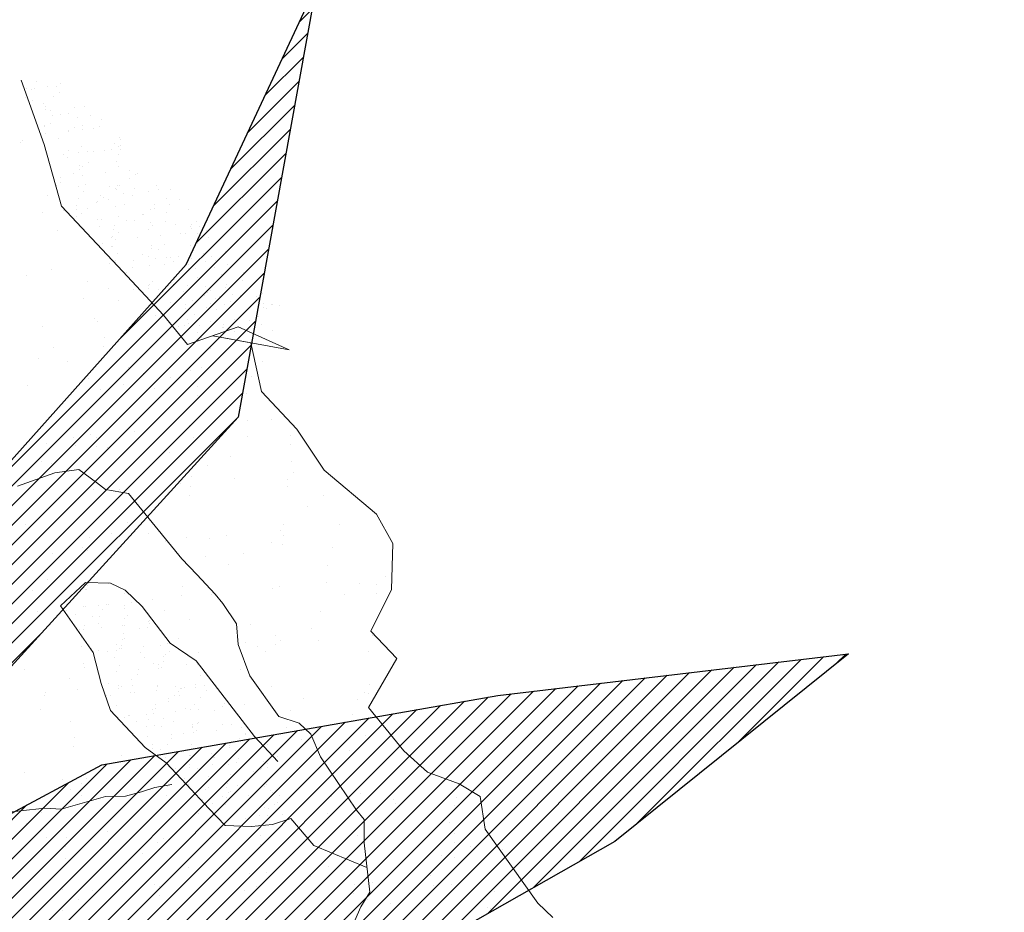
# Model space of a CAD drawing. Units: inches. Extents: x 1986 to 21484, y -1816 to 2016.
# Tile 75 of 85: x 3676.66 to 3687.55, y 1888.79 to 1898.67. Entities that reach past the tile are written whole.
import ezdxf

# ---------------------------------------------------------------- set-up
doc = ezdxf.new("R2010")
doc.units = ezdxf.units.IN
doc.layers.add('L-PLNT', color=84, linetype='Continuous', lineweight=13)
doc.layers.add('vfolhas', color=114, linetype='Continuous', lineweight=5)
doc.layers.add('vfolha2', color=110, linetype='Continuous')
doc.layers.add('vfolhas2', color=102, linetype='Continuous')
pattern_1 = [(45, (-2446.5133113, 50.986076), (-0.004419417382, 0.004419417382), [])]

# ---------------------------------------------------------------- blocks, each defined once
blk = doc.blocks.new('arbusto_PB_verde_grande')
at = {"layer": 'vfolha2'}
h = blk.add_hatch(dxfattribs=at)
h.set_pattern_fill('ANSI31', color=256, scale=0.05, style=0)
h.set_pattern_definition(pattern_1)
h.paths.add_polyline_path([(0.02944, 0.35651), (0.00028, 0.09048), (0.02625, -0.03934), (0.047, 0.06233), (0.06189, 0.09731), (0.09372, 0.26573), (0.09955, 0.43473), (0.08789, 0.61313), (0.0645, 0.72266), (0.04988, 0.6851), (0.0236, 0.51294)])
h.paths.add_polyline_path([(0.30106, 0.43789), (0.14225, 0.24871), (0.26685, 0.30022)])
h.paths.add_polyline_path([(0.37995, 0.22817), (0.23697, 0.15193), (0.18428, 0.09364), (0.11122, 0.04358), (0.02625, -0.03934), (0.28061, 0.04667), (0.36829, 0.07798), (0.46756, 0.11239), (0.61068, 0.19376), (0.71585, 0.27823), (0.55813, 0.25948)])
h.paths.add_polyline_path([(0.56101, -0.29441), (0.72752, -0.32573), (0.59024, -0.2412), (0.42962, -0.15982), (0.02625, -0.03934), (0.14922, -0.14107), (0.18838, -0.16604), (0.41501, -0.24435)])
h.paths.add_polyline_path([(-0.27429, -0.44776), (-0.30352, -0.72628), (-0.23923, -0.64175), (-0.15457, -0.45716), (0.02625, -0.03934), (-0.16328, -0.25376)])
h.paths.add_polyline_path([(-0.51963, -0.24744), (-0.67736, -0.32573), (-0.59558, -0.35072), (-0.40574, -0.32882), (-0.21007, -0.20995), (0.02625, -0.03934), (-0.14874, -0.06595), (-0.31518, -0.09101), (-0.41452, -0.15048)])
h.paths.add_polyline_path([(-0.52546, 0.25007), (-0.70947, 0.24698), (-0.51963, 0.1093), (-0.32979, 0.02167), (-0.07567, -0.0128), (-0.04234, -0.02148), (-0.35024, 0.1312)])
at = {"layer": 'vfolhas'}
h = blk.add_hatch(dxfattribs=at)
h.set_pattern_fill('ANSI31', color=256, scale=0.05, style=0)
h.set_pattern_definition(pattern_1)
h.paths.add_polyline_path([(-0.07279, 0.50669), (-0.18085, 0.65063), (-0.2334, 0.67253), (-0.20712, 0.53176), (-0.10785, 0.25007), (0.02625, -0.03934), (0.00028, 0.09048), (0.00816, 0.16241), (-0.04939, 0.29079)])
h.paths.add_polyline_path([(0.09902, 0.41929), (0.09372, 0.26573), (0.07906, 0.18814), (0.15506, 0.36901), (0.26606, 0.5505), (0.28356, 0.63504), (0.2485, 0.68819), (0.25145, 0.63504), (0.20178, 0.54426)])
h.paths.add_polyline_path([(0.12295, 0.24073), (0.047, 0.06233), (0.02625, -0.03934), (0.11122, 0.04358), (0.18428, 0.09364), (0.27478, 0.19376), (0.3215, 0.25323), (0.44129, 0.38467), (0.47634, 0.57866), (0.41789, 0.45347), (0.28939, 0.30954)])
h.paths.add_polyline_path([(0.58145, -0.03779), (0.70707, 0.01536), (0.78591, 0.04667), (0.74796, 0.06549), (0.62818, 0.08423), (0.52595, 0.09048), (0.39745, 0.04358), (0.02625, -0.03934), (0.25728, -0.03154), (0.43834, -0.0347)])
h.paths.add_polyline_path([(0.52022, -0.03647), (0.43834, -0.0347), (0.25728, -0.03154), (0.02625, -0.03934), (0.17964, -0.08515), (0.53768, -0.13167), (0.69541, -0.15357), (0.78591, -0.07852), (0.70413, -0.10042)])
h.paths.add_polyline_path([(0.27189, -0.21929), (0.14922, -0.14107), (0.02625, -0.03934), (0.15794, -0.31007), (0.29522, -0.42585), (0.41789, -0.49157), (0.56396, -0.56669), (0.5114, -0.48532), (0.39456, -0.34139)])
h.paths.add_polyline_path([(-0.05818, -0.47591), (-0.02312, -0.61984), (0.047, -0.80134), (0.08494, -0.59794), (0.07911, -0.4071), (0.03527, -0.25376), (0.02625, -0.03934), (-0.03773, -0.26001)])
h.paths.add_polyline_path([(-0.24218, 0.14054), (-0.11073, 0.06858), (0.02625, -0.03934), (-0.04235, 0.10871), (-0.21007, 0.23757), (-0.36485, 0.33145), (-0.47874, 0.40341), (-0.54303, 0.46288), (-0.49041, 0.33145), (-0.39408, 0.22192)])
at = {"layer": 'vfolha2'}
for p, q in [((0.55813, 0.25948), (0.71585, 0.27823)), ((0.71585, 0.27823), (0.61068, 0.19376)), ((0.37995, 0.22817), (0.55813, 0.25948)), ((0.23697, 0.15193), (0.37995, 0.22817)), ((0.61068, 0.19376), (0.46756, 0.11239))]:
    blk.add_line(p, q, dxfattribs=at)
at = {"layer": 'vfolhas2'}
for p, q in [((0.41789, 0.45347), (0.47634, 0.57866)), ((0.47634, 0.57866), (0.44129, 0.38467)), ((0.28939, 0.30954), (0.41789, 0.45347)), ((0.44129, 0.38467), (0.3215, 0.25323))]:
    blk.add_line(p, q, dxfattribs=at)
blk = doc.blocks.new('PLANT-SHRUB')
for p, q in [((2150.827, 1895.541), (2150.816, 1895.77)), ((2150.691, 1894.545), (2150.827, 1895.541)), ((2151.251, 1895.226), (2151.251, 1895.226)), ((2151.271, 1895.193), (2151.271, 1895.193)), ((2151.082, 1895.119), (2151.082, 1895.119)), ((2150.707, 1894.836), (2150.707, 1894.836)), ((2151.387, 1894.734), (2151.387, 1894.734)), ((2150.482, 1894.243), (2150.691, 1894.545)), ((2150.945, 1894.573), (2150.945, 1894.573)), ((2151.153, 1894.546), (2151.153, 1894.546)), ((2151.535, 1894.612), (2151.535, 1894.612)), ((2151.246, 1894.423), (2151.246, 1894.423)), ((2151.478, 1894.503), (2151.478, 1894.503)), ((2152.021, 1894.431), (2152.021, 1894.431)), ((2152.282, 1894.23), (2152.778, 1894.439)), ((2150.966, 1894.348), (2150.966, 1894.348)), ((2151.039, 1894.416), (2151.039, 1894.416)), ((2150.555, 1893.982), (2150.482, 1894.243)), ((2150.928, 1894.225), (2150.928, 1894.225)), ((2152.099, 1894.178), (2152.282, 1894.23)), ((2152.173, 1894.223), (2152.173, 1894.223)), ((2150.76, 1894.118), (2150.76, 1894.118)), ((2151.771, 1893.736), (2152.099, 1894.178)), ((2152.004, 1894.116), (2152.004, 1894.116)), ((2150.722, 1893.648), (2150.555, 1893.982)), ((2150.568, 1893.984), (2150.568, 1893.984)), ((2150.682, 1894.066), (2150.682, 1894.066)), ((2151.761, 1894.027), (2151.761, 1894.027)), ((2152.167, 1893.998), (2152.167, 1893.998)), ((2152.241, 1894.065), (2152.241, 1894.065)), ((2151.935, 1893.957), (2152.198, 1893.378)), ((2151.595, 1893.55), (2151.771, 1893.736)), ((2152.243, 1893.657), (2152.243, 1893.657)), ((2150.753, 1893.294), (2150.722, 1893.648)), ((2151.212, 1893.611), (2151.212, 1893.611)), ((2151.221, 1893.652), (2151.221, 1893.652)), ((2151.585, 1893.416), (2151.595, 1893.55)), ((2151.769, 1893.633), (2151.769, 1893.633)), ((2152.457, 1893.609), (2152.457, 1893.609)), ((2151.471, 1892.713), (2151.585, 1893.416)), ((2152.198, 1893.378), (2152.179, 1892.988)), ((2150.712, 1892.679), (2150.753, 1893.294)), ((2151.348, 1893.247), (2151.348, 1893.247)), ((2151.422, 1893.314), (2151.422, 1893.314)), ((2151.736, 1893.257), (2151.736, 1893.257)), ((2151.85, 1893.222), (2151.85, 1893.222)), ((2152.782, 1893.244), (2152.782, 1893.244)), ((2152.971, 1893.282), (2152.971, 1893.282)), ((2153.095, 1893.22), (2153.095, 1893.22)), ((2151.681, 1893.115), (2151.681, 1893.115)), ((2152.926, 1893.113), (2152.926, 1893.113)), ((2152.179, 1892.988), (2152.372, 1892.896)), ((2152.372, 1892.896), (2152.555, 1892.753)), ((2152.55, 1892.896), (2152.55, 1892.896)), ((2152.623, 1892.964), (2152.623, 1892.964)), ((2150.95, 1892.882), (2150.95, 1892.882)), ((2151.195, 1892.882), (2151.195, 1892.882)), ((2152.218, 1892.887), (2152.218, 1892.887)), ((2152.218, 1892.887), (2152.218, 1892.887)), ((2152.35, 1892.786), (2152.35, 1892.786)), ((2152.445, 1892.82), (2152.445, 1892.82)), ((2153.297, 1892.848), (2153.297, 1892.848)), ((2150.111, 1892.499), (2150.712, 1892.679)), ((2151.378, 1892.455), (2151.471, 1892.713)), ((2152.096, 1892.714), (2152.096, 1892.714)), ((2152.164, 1892.757), (2152.164, 1892.757)), ((2152.202, 1892.752), (2152.202, 1892.752)), ((2152.285, 1892.741), (2152.285, 1892.741)), ((2152.306, 1892.693), (2152.306, 1892.693)), ((2152.415, 1892.724), (2152.415, 1892.724)), ((2152.555, 1892.753), (2152.763, 1892.545)), ((2152.594, 1892.713), (2152.594, 1892.713)), ((2150.603, 1892.564), (2150.603, 1892.564)), ((2150.889, 1892.61), (2150.889, 1892.61)), ((2152.134, 1892.636), (2152.134, 1892.636)), ((2152.134, 1892.608), (2152.134, 1892.608)), ((2152.134, 1892.608), (2152.134, 1892.608)), ((2152.277, 1892.666), (2152.277, 1892.666)), ((2152.543, 1892.638), (2152.543, 1892.638)), ((2153.379, 1892.606), (2153.379, 1892.606)), ((2153.825, 1892.613), (2153.825, 1892.613)), ((2150.111, 1892.079), (2150.111, 1892.499)), ((2150.529, 1892.496), (2150.529, 1892.496)), ((2150.631, 1892.526), (2150.631, 1892.526)), ((2150.741, 1892.53), (2150.741, 1892.53)), ((2151.284, 1892.459), (2151.284, 1892.459)), ((2151.711, 1892.487), (2151.711, 1892.487)), ((2151.909, 1892.493), (2151.909, 1892.493)), ((2152.117, 1892.52), (2152.117, 1892.52)), ((2152.152, 1892.532), (2152.152, 1892.532)), ((2152.152, 1892.532), (2152.152, 1892.532)), ((2152.277, 1892.511), (2152.277, 1892.511)), ((2152.34, 1892.478), (2152.34, 1892.478)), ((2152.757, 1892.526), (2152.757, 1892.526)), ((2152.757, 1892.474), (2152.757, 1892.474)), ((2152.757, 1892.474), (2152.757, 1892.474)), ((2152.759, 1892.472), (2152.759, 1892.472)), ((2152.763, 1892.545), (2152.763, 1892.284)), ((2153.751, 1892.545), (2153.751, 1892.545)), ((2153.779, 1892.479), (2153.779, 1892.479)), ((2151.388, 1892.279), (2151.378, 1892.455)), ((2151.492, 1892.431), (2151.492, 1892.431)), ((2151.817, 1892.389), (2151.817, 1892.389)), ((2151.851, 1892.427), (2151.851, 1892.427)), ((2151.851, 1892.05), (2151.851, 1892.427)), ((2151.949, 1892.366), (2151.949, 1892.366)), ((2151.978, 1892.393), (2151.978, 1892.393)), ((2152.035, 1892.357), (2152.035, 1892.357)), ((2152.054, 1892.357), (2152.054, 1892.357)), ((2152.137, 1892.346), (2152.137, 1892.346)), ((2152.532, 1892.356), (2152.532, 1892.356)), ((2152.598, 1892.38), (2152.598, 1892.38)), ((2151.502, 1892.072), (2151.388, 1892.279)), ((2151.967, 1892.314), (2151.967, 1892.314)), ((2152.124, 1892.328), (2152.124, 1892.328)), ((2152.267, 1892.329), (2152.267, 1892.329)), ((2152.36, 1892.317), (2152.36, 1892.317)), ((2152.36, 1892.317), (2152.36, 1892.317)), ((2152.459, 1892.252), (2152.459, 1892.252)), ((2152.465, 1892.313), (2152.465, 1892.313)), ((2152.485, 1892.301), (2152.485, 1892.301)), ((2152.533, 1892.33), (2152.533, 1892.33)), ((2152.568, 1892.29), (2152.568, 1892.29)), ((2152.568, 1892.29), (2152.568, 1892.29)), ((2152.568, 1892.29), (2152.568, 1892.29)), ((2152.698, 1892.273), (2152.698, 1892.273)), ((2152.763, 1892.284), (2152.763, 1891.92)), ((2152.893, 1892.247), (2152.893, 1892.247)), ((2150.131, 1892.132), (2150.131, 1892.132)), ((2150.283, 1892.224), (2150.283, 1892.224)), ((2151.527, 1892.221), (2151.527, 1892.221)), ((2151.73, 1892.146), (2151.73, 1892.146)), ((2151.804, 1892.213), (2151.804, 1892.213)), ((2151.898, 1892.185), (2151.898, 1892.185)), ((2152.33, 1892.17), (2152.33, 1892.17)), ((2152.429, 1892.225), (2152.429, 1892.225)), ((2152.749, 1892.164), (2152.749, 1892.164)), ((2152.772, 1892.219), (2152.772, 1892.219)), ((2153.353, 1892.181), (2153.353, 1892.181)), ((2153.436, 1892.175), (2153.436, 1892.175)), ((2153.644, 1892.148), (2153.644, 1892.148)), ((2154.016, 1892.217), (2154.016, 1892.217)), ((2149.63, 1891.899), (2150.111, 1892.079)), ((2150.114, 1892.116), (2150.114, 1892.116)), ((2150.124, 1892.126), (2150.124, 1892.126)), ((2151.17, 1892.112), (2151.17, 1892.112)), ((2151.359, 1892.114), (2151.359, 1892.114)), ((2151.429, 1891.525), (2151.502, 1892.072)), ((2151.747, 1890.995), (2151.851, 1892.05)), ((2151.851, 1892.05), (2151.851, 1892.05)), ((2152.114, 1892.02), (2152.114, 1892.02)), ((2152.148, 1892.111), (2152.148, 1892.111)), ((2152.193, 1892.117), (2152.193, 1892.117)), ((2152.193, 1892.117), (2152.193, 1892.117)), ((2152.27, 1892.08), (2152.27, 1892.08)), ((2152.523, 1892.022), (2152.523, 1892.022)), ((2152.603, 1892.112), (2152.603, 1892.112)), ((2152.603, 1892.112), (2152.603, 1892.112)), ((2152.646, 1892.11), (2152.646, 1892.11)), ((2153.272, 1892.078), (2153.272, 1892.078)), ((2153.848, 1892.11), (2153.848, 1892.11)), ((2153.969, 1892.105), (2153.969, 1892.105)), ((2154.318, 1892.065), (2154.318, 1892.065)), ((2154.511, 1892.034), (2154.511, 1892.034)), ((2151.838, 1891.914), (2151.838, 1891.914)), ((2151.905, 1891.956), (2151.905, 1891.956)), ((2151.907, 1891.963), (2151.907, 1891.963)), ((2151.99, 1891.952), (2151.99, 1891.952)), ((2152.102, 1891.925), (2152.102, 1891.925)), ((2152.12, 1891.935), (2152.12, 1891.935)), ((2152.131, 1891.952), (2152.131, 1891.952)), ((2152.336, 1891.913), (2152.336, 1891.913)), ((2152.403, 1891.956), (2152.403, 1891.956)), ((2152.751, 1891.939), (2152.751, 1891.939)), ((2152.763, 1891.92), (2152.763, 1891.594)), ((2154.719, 1892.006), (2154.719, 1892.006)), ((2149.27, 1891.538), (2149.63, 1891.899)), ((2149.783, 1891.813), (2149.783, 1891.813)), ((2151.888, 1891.877), (2151.888, 1891.877)), ((2152.32, 1891.861), (2152.32, 1891.861)), ((2152.337, 1891.906), (2152.337, 1891.906)), ((2152.42, 1891.895), (2152.42, 1891.895)), ((2152.55, 1891.878), (2152.55, 1891.878)), ((2152.612, 1891.812), (2152.612, 1891.812)), ((2152.739, 1891.856), (2152.739, 1891.856)), ((2152.88, 1891.812), (2153.043, 1891.706)), ((2153.006, 1891.862), (2153.006, 1891.862)), ((2154.555, 1891.83), (2154.555, 1891.83)), ((2149.584, 1891.751), (2149.584, 1891.751)), ((2149.71, 1891.746), (2149.71, 1891.746)), ((2150.606, 1891.756), (2150.606, 1891.756)), ((2151.333, 1891.781), (2151.333, 1891.781)), ((2151.686, 1891.717), (2151.686, 1891.717)), ((2151.943, 1891.779), (2151.943, 1891.779)), ((2152.019, 1891.711), (2152.019, 1891.711)), ((2152.104, 1891.712), (2152.104, 1891.712)), ((2152.513, 1891.714), (2152.513, 1891.714)), ((2152.517, 1891.71), (2152.517, 1891.71)), ((2152.582, 1891.785), (2152.582, 1891.785)), ((2152.732, 1891.704), (2152.732, 1891.704)), ((2152.732, 1891.704), (2152.732, 1891.704)), ((2152.932, 1891.795), (2152.932, 1891.795)), ((2153.043, 1891.706), (2153.181, 1891.641)), ((2153.754, 1891.708), (2153.754, 1891.708)), ((2149.84, 1891.614), (2149.84, 1891.614)), ((2150.048, 1891.587), (2150.048, 1891.587)), ((2150.567, 1891.609), (2150.567, 1891.609)), ((2151.811, 1891.607), (2151.811, 1891.607)), ((2151.811, 1891.607), (2151.811, 1891.607)), ((2152.423, 1891.639), (2152.423, 1891.639)), ((2152.763, 1891.594), (2152.815, 1891.308)), ((2153.056, 1891.605), (2153.056, 1891.605)), ((2153.181, 1891.641), (2153.344, 1891.552)), ((2154.3, 1891.603), (2154.3, 1891.603)), ((2154.834, 1891.67), (2154.834, 1891.67)), ((2149.179, 1891.178), (2149.27, 1891.538)), ((2150.373, 1891.544), (2150.373, 1891.544)), ((2151.285, 1891.184), (2151.429, 1891.525)), ((2151.843, 1891.557), (2151.843, 1891.557)), ((2151.878, 1891.569), (2151.878, 1891.569)), ((2151.973, 1891.54), (2151.973, 1891.54)), ((2152.19, 1891.512), (2152.19, 1891.512)), ((2152.207, 1891.512), (2152.207, 1891.512)), ((2152.255, 1891.485), (2152.255, 1891.485)), ((2152.273, 1891.501), (2152.273, 1891.501)), ((2152.274, 1891.555), (2152.274, 1891.555)), ((2152.284, 1891.512), (2152.284, 1891.512)), ((2152.31, 1891.553), (2152.31, 1891.553)), ((2152.403, 1891.484), (2152.403, 1891.484)), ((2152.705, 1891.511), (2152.705, 1891.511)), ((2152.729, 1891.548), (2152.729, 1891.548)), ((2153.344, 1891.552), (2153.506, 1891.405)), ((2154.207, 1891.511), (2154.207, 1891.511)), ((2150.911, 1891.395), (2150.911, 1891.395)), ((2150.915, 1891.472), (2150.915, 1891.472)), ((2150.985, 1891.462), (2150.985, 1891.462)), ((2151.123, 1891.445), (2151.123, 1891.445)), ((2151.448, 1891.402), (2151.448, 1891.402)), ((2152.094, 1891.404), (2152.094, 1891.404)), ((2152.503, 1891.406), (2152.503, 1891.406)), ((2152.534, 1891.43), (2152.534, 1891.43)), ((2152.534, 1891.43), (2152.534, 1891.43)), ((2152.62, 1891.455), (2152.62, 1891.455)), ((2152.703, 1891.444), (2152.703, 1891.444)), ((2152.765, 1891.371), (2152.765, 1891.371)), ((2153.506, 1891.405), (2153.962, 1891.17)), ((2154.133, 1891.444), (2154.133, 1891.444)), ((2150.099, 1891.356), (2150.099, 1891.356)), ((2151.145, 1891.342), (2151.145, 1891.342)), ((2151.868, 1891.261), (2151.868, 1891.261)), ((2151.89, 1891.31), (2151.89, 1891.31)), ((2151.991, 1891.331), (2151.991, 1891.331)), ((2151.991, 1891.331), (2151.991, 1891.331)), ((2152.096, 1891.339), (2152.096, 1891.339)), ((2152.167, 1891.347), (2152.167, 1891.347)), ((2152.167, 1891.347), (2152.167, 1891.347)), ((2152.199, 1891.303), (2152.199, 1891.303)), ((2152.199, 1891.303), (2152.199, 1891.303)), ((2152.388, 1891.31), (2152.388, 1891.31)), ((2152.524, 1891.261), (2152.524, 1891.261)), ((2152.524, 1891.261), (2152.524, 1891.261)), ((2152.735, 1891.344), (2152.735, 1891.344)), ((2152.815, 1891.308), (2152.815, 1890.748)), ((2153.247, 1891.308), (2153.247, 1891.308)), ((2154.293, 1891.295), (2154.293, 1891.295)), ((2149.27, 1890.427), (2149.179, 1891.178)), ((2149.96, 1891.223), (2149.96, 1891.223)), ((2151.14, 1891.004), (2151.285, 1891.184)), ((2151.204, 1891.221), (2151.204, 1891.221)), ((2151.927, 1891.184), (2151.927, 1891.184)), ((2151.957, 1891.211), (2151.957, 1891.211)), ((2152.145, 1891.155), (2152.145, 1891.155)), ((2152.3, 1891.245), (2152.3, 1891.245)), ((2152.449, 1891.218), (2152.449, 1891.218)), ((2152.449, 1891.218), (2152.449, 1891.218)), ((2152.576, 1891.199), (2152.576, 1891.199)), ((2152.643, 1891.154), (2152.643, 1891.154)), ((2152.718, 1891.24), (2152.718, 1891.24)), ((2153.067, 1891.189), (2153.067, 1891.189)), ((2153.275, 1891.162), (2153.275, 1891.162)), ((2153.694, 1891.216), (2153.694, 1891.216)), ((2153.962, 1891.17), (2154.084, 1891.04)), ((2149.791, 1891.116), (2149.791, 1891.116)), ((2151.036, 1891.113), (2151.036, 1891.113)), ((2151.768, 1891.039), (2151.768, 1891.039)), ((2151.825, 1891.146), (2151.825, 1891.146)), ((2152.042, 1891.117), (2152.042, 1891.117)), ((2152.078, 1891.112), (2152.078, 1891.112)), ((2152.084, 1891.096), (2152.084, 1891.096)), ((2152.113, 1891.044), (2152.113, 1891.044)), ((2152.113, 1891.044), (2152.113, 1891.044)), ((2152.126, 1891.106), (2152.126, 1891.106)), ((2152.186, 1891.112), (2152.186, 1891.112)), ((2152.186, 1891.112), (2152.186, 1891.112)), ((2152.256, 1891.089), (2152.256, 1891.089)), ((2152.281, 1891.111), (2152.281, 1891.111)), ((2152.281, 1891.111), (2152.281, 1891.111)), ((2152.408, 1891.044), (2152.408, 1891.044)), ((2152.437, 1891.071), (2152.437, 1891.071)), ((2152.473, 1891.06), (2152.473, 1891.06)), ((2152.493, 1891.097), (2152.493, 1891.097)), ((2152.556, 1891.049), (2152.556, 1891.049)), ((2152.575, 1891.111), (2152.575, 1891.111)), ((2153.525, 1891.109), (2153.525, 1891.109)), ((2153.6, 1891.119), (2153.6, 1891.119)), ((2153.736, 1891.079), (2153.736, 1891.079)), ((2154.084, 1891.04), (2154.303, 1890.877)), ((2154.143, 1891.048), (2154.143, 1891.048)), ((2149.558, 1890.981), (2149.558, 1890.981)), ((2150.513, 1891.03), (2150.513, 1891.03)), ((2150.581, 1890.986), (2150.581, 1890.986)), ((2151.099, 1890.736), (2151.14, 1891.004)), ((2151.66, 1890.947), (2151.66, 1890.947)), ((2151.825, 1890.657), (2151.747, 1890.995)), ((2151.858, 1890.953), (2151.858, 1890.953)), ((2152.29, 1890.937), (2152.29, 1890.937)), ((2152.686, 1891.032), (2152.686, 1891.032)), ((2152.707, 1890.933), (2152.707, 1890.933)), ((2152.707, 1890.933), (2152.707, 1890.933)), ((2152.708, 1890.932), (2152.708, 1890.932)), ((2153.729, 1890.938), (2153.729, 1890.938)), ((2154.351, 1891.02), (2154.351, 1891.02)), ((2152.249, 1890.898), (2152.249, 1890.898)), ((2152.259, 1890.909), (2152.259, 1890.909)), ((2152.756, 1890.908), (2152.756, 1890.908)), ((2154.303, 1890.877), (2154.547, 1890.698)), ((2150.166, 1890.712), (2150.166, 1890.712)), ((2151.088, 1890.601), (2151.099, 1890.736)), ((2151.895, 1890.723), (2151.895, 1890.723)), ((2151.949, 1890.712), (2151.949, 1890.712)), ((2151.978, 1890.712), (2151.978, 1890.712)), ((2152.016, 1890.755), (2152.016, 1890.755)), ((2152.074, 1890.787), (2152.074, 1890.787)), ((2152.08, 1890.744), (2152.08, 1890.744)), ((2152.109, 1890.771), (2152.109, 1890.771)), ((2152.483, 1890.789), (2152.483, 1890.789)), ((2152.514, 1890.754), (2152.514, 1890.754)), ((2152.815, 1890.748), (2152.685, 1890.461)), ((2152.729, 1890.758), (2152.729, 1890.758)), ((2153.388, 1890.761), (2153.388, 1890.761)), ((2149.471, 1890.628), (2149.471, 1890.628)), ((2150.092, 1890.644), (2150.092, 1890.644)), ((2150.244, 1890.609), (2150.244, 1890.609)), ((2151.488, 1890.606), (2151.488, 1890.606)), ((2151.715, 1890.68), (2151.715, 1890.68)), ((2151.773, 1890.149), (2151.825, 1890.657)), ((2151.848, 1890.645), (2151.848, 1890.645)), ((2152.108, 1890.695), (2152.108, 1890.695)), ((2152.28, 1890.629), (2152.28, 1890.629)), ((2152.325, 1890.666), (2152.325, 1890.666)), ((2152.408, 1890.655), (2152.408, 1890.655)), ((2152.446, 1890.711), (2152.446, 1890.711)), ((2152.538, 1890.638), (2152.538, 1890.638)), ((2152.561, 1890.604), (2152.561, 1890.604)), ((2152.59, 1890.631), (2152.59, 1890.631)), ((2152.698, 1890.624), (2152.698, 1890.624)), ((2152.733, 1890.604), (2152.733, 1890.604)), ((2152.733, 1890.604), (2152.733, 1890.604)), ((2153.314, 1890.693), (2153.314, 1890.693)), ((2149.679, 1890.6), (2149.679, 1890.6)), ((2150.004, 1890.558), (2150.004, 1890.558)), ((2150.074, 1890.585), (2150.074, 1890.585)), ((2151.088, 1890.302), (2151.088, 1890.601)), ((2151.12, 1890.572), (2151.12, 1890.572)), ((2151.921, 1890.598), (2151.921, 1890.598)), ((2152.13, 1890.509), (2152.13, 1890.509)), ((2152.142, 1890.577), (2152.142, 1890.577)), ((2152.142, 1890.577), (2152.142, 1890.577)), ((2152.627, 1890.508), (2152.627, 1890.508)), ((2153.222, 1890.538), (2153.222, 1890.538)), ((2153.978, 1890.602), (2153.978, 1890.602)), ((2149.179, 1889.886), (2149.27, 1890.427)), ((2150.547, 1890.486), (2150.547, 1890.486)), ((2150.755, 1890.459), (2150.755, 1890.459)), ((2151.08, 1890.416), (2151.08, 1890.416)), ((2152.064, 1890.479), (2152.064, 1890.479)), ((2152.401, 1890.458), (2152.401, 1890.458)), ((2152.473, 1890.481), (2152.473, 1890.481)), ((2152.685, 1890.461), (2152.516, 1890.149)), ((2152.685, 1890.461), (2152.685, 1890.461)), ((2149.694, 1890.28), (2149.694, 1890.28)), ((2151.088, 1890.064), (2151.088, 1890.302)), ((2151.293, 1890.293), (2151.293, 1890.293)), ((2151.367, 1890.361), (2151.367, 1890.361)), ((2151.623, 1890.345), (2151.623, 1890.345)), ((2151.819, 1890.311), (2151.819, 1890.311)), ((2151.831, 1890.317), (2151.831, 1890.317)), ((2151.831, 1890.317), (2151.831, 1890.317)), ((2151.831, 1890.317), (2151.831, 1890.317)), ((2151.838, 1890.337), (2151.838, 1890.337)), ((2151.887, 1890.354), (2151.887, 1890.354)), ((2151.961, 1890.3), (2151.961, 1890.3)), ((2152.233, 1890.303), (2152.233, 1890.303)), ((2152.262, 1890.33), (2152.262, 1890.33)), ((2152.27, 1890.321), (2152.27, 1890.321)), ((2152.317, 1890.31), (2152.317, 1890.31)), ((2152.385, 1890.353), (2152.385, 1890.353)), ((2152.916, 1890.329), (2152.916, 1890.329)), ((2149.533, 1890.211), (2149.533, 1890.211)), ((2149.637, 1890.222), (2149.637, 1890.222)), ((2150.556, 1890.216), (2150.556, 1890.216)), ((2150.882, 1890.22), (2150.882, 1890.22)), ((2151.635, 1890.177), (2151.635, 1890.177)), ((2152.054, 1890.171), (2152.054, 1890.171)), ((2152.126, 1890.218), (2152.126, 1890.218)), ((2152.126, 1890.218), (2152.126, 1890.218)), ((2152.156, 1890.274), (2152.156, 1890.274)), ((2152.156, 1890.274), (2152.156, 1890.274)), ((2152.178, 1890.271), (2152.178, 1890.271)), ((2152.261, 1890.26), (2152.261, 1890.26)), ((2152.391, 1890.243), (2152.391, 1890.243)), ((2152.463, 1890.173), (2152.463, 1890.173)), ((2152.699, 1890.203), (2152.699, 1890.203)), ((2152.907, 1890.175), (2152.907, 1890.175)), ((2153.371, 1890.215), (2153.371, 1890.215)), ((2149.468, 1890.115), (2149.468, 1890.115)), ((2150.713, 1890.112), (2150.713, 1890.112)), ((2151.026, 1889.131), (2151.088, 1890.064)), ((2151.786, 1889.889), (2151.773, 1890.149)), ((2151.958, 1890.11), (2151.958, 1890.11)), ((2151.958, 1890.11), (2151.958, 1890.11)), ((2152, 1890.109), (2152, 1890.109)), ((2152.074, 1890.157), (2152.074, 1890.157)), ((2152.516, 1890.149), (2152.424, 1889.524)), ((2152.498, 1890.108), (2152.498, 1890.108)), ((2152.681, 1890.163), (2152.681, 1890.163)), ((2153.202, 1890.108), (2153.202, 1890.108)), ((2153.232, 1890.133), (2153.232, 1890.133)), ((2149.347, 1889.961), (2149.347, 1889.961)), ((2151.828, 1890.029), (2151.828, 1890.029)), ((2151.905, 1890.003), (2151.905, 1890.003)), ((2151.935, 1890.03), (2151.935, 1890.03)), ((2152.256, 1889.953), (2152.256, 1889.953)), ((2152.26, 1890.013), (2152.26, 1890.013)), ((2152.569, 1890.01), (2152.569, 1890.01)), ((2149.179, 1889.886), (2149.179, 1889.886)), ((2149.179, 1889.316), (2149.179, 1889.886)), ((2149.273, 1889.894), (2149.273, 1889.894)), ((2150.896, 1889.929), (2150.896, 1889.929)), ((2151.851, 1889.719), (2151.786, 1889.889)), ((2151.813, 1889.905), (2151.813, 1889.905)), ((2152.03, 1889.877), (2152.03, 1889.877)), ((2152.044, 1889.863), (2152.044, 1889.863)), ((2152.114, 1889.866), (2152.114, 1889.866)), ((2152.188, 1889.91), (2152.188, 1889.91)), ((2152.244, 1889.849), (2152.244, 1889.849)), ((2152.386, 1889.863), (2152.386, 1889.863)), ((2152.415, 1889.89), (2152.415, 1889.89)), ((2152.453, 1889.865), (2152.453, 1889.865)), ((2152.495, 1889.943), (2152.495, 1889.943)), ((2150.049, 1889.815), (2150.049, 1889.815)), ((2151.095, 1889.802), (2151.095, 1889.802)), ((2152.117, 1889.807), (2152.117, 1889.807)), ((2152.117, 1889.807), (2152.117, 1889.807)), ((2152.461, 1889.82), (2152.461, 1889.82)), ((2153.197, 1889.768), (2153.197, 1889.768)), ((2152.047, 1889.524), (2151.851, 1889.719)), ((2151.871, 1889.708), (2151.871, 1889.708)), ((2152.227, 1889.717), (2152.227, 1889.717)), ((2152.25, 1889.705), (2152.25, 1889.705)), ((2152.369, 1889.707), (2152.369, 1889.707)), ((2149.311, 1889.614), (2149.311, 1889.614)), ((2149.636, 1889.571), (2149.636, 1889.571)), ((2149.921, 1889.608), (2149.921, 1889.608)), ((2150.474, 1889.543), (2150.474, 1889.543)), ((2150.548, 1889.61), (2150.548, 1889.61)), ((2151.166, 1889.606), (2151.166, 1889.606)), ((2152.034, 1889.555), (2152.034, 1889.555)), ((2152.047, 1889.524), (2152.047, 1889.524)), ((2152.424, 1889.524), (2152.047, 1889.524)), ((2152.058, 1889.562), (2152.058, 1889.562)), ((2152.088, 1889.589), (2152.088, 1889.589)), ((2152.097, 1889.578), (2152.097, 1889.578)), ((2152.097, 1889.578), (2152.097, 1889.578)), ((2152.126, 1889.553), (2152.126, 1889.553)), ((2152.41, 1889.603), (2152.41, 1889.603)), ((2152.41, 1889.603), (2152.41, 1889.603)), ((2152.424, 1889.524), (2152.424, 1889.524)), ((2149.508, 1889.441), (2149.508, 1889.441)), ((2150.178, 1889.5), (2150.178, 1889.5)), ((2150.386, 1889.472), (2150.386, 1889.472)), ((2150.531, 1889.446), (2150.531, 1889.446)), ((2150.711, 1889.43), (2150.711, 1889.43)), ((2151.61, 1889.407), (2151.61, 1889.407)), ((2148.894, 1888.843), (2149.179, 1889.316)), ((2151.254, 1889.358), (2151.254, 1889.358)), ((2151.462, 1889.331), (2151.462, 1889.331)), ((2152.656, 1889.393), (2152.656, 1889.393)), ((2148.639, 1889.189), (2149.15, 1888.498)), ((2148.639, 1889.189), (2148.879, 1888.618)), ((2149.314, 1889.221), (2149.314, 1889.221)), ((2150.559, 1889.219), (2150.559, 1889.219)), ((2151.676, 1889.192), (2151.676, 1889.192)), ((2151.749, 1889.26), (2151.749, 1889.26)), ((2151.787, 1889.288), (2151.787, 1889.288)), ((2151.803, 1889.217), (2151.803, 1889.217)), ((2152.33, 1889.217), (2152.33, 1889.217)), ((2152.538, 1889.189), (2152.538, 1889.189)), ((2148.944, 1889.084), (2148.944, 1889.084)), ((2149.146, 1889.114), (2149.146, 1889.114)), ((2150.077, 1889.178), (2150.077, 1889.178)), ((2150.39, 1889.112), (2150.39, 1889.112)), ((2151.026, 1889.131), (2151.026, 1889.131)), ((2151.181, 1888.925), (2151.026, 1889.131)), ((2151.635, 1889.109), (2151.635, 1889.109)), ((2150.023, 1889.045), (2150.023, 1889.045)), ((2151.07, 1889.032), (2151.07, 1889.032)), ((2152.092, 1889.037), (2152.092, 1889.037)), ((2148.626, 1888.913), (2148.626, 1888.913)), ((2149.729, 1888.86), (2149.729, 1888.86)), ((2151.181, 1888.925), (2151.181, 1888.925)), ((2151.202, 1888.801), (2151.181, 1888.925)), ((2148.383, 1888.758), (2148.383, 1888.758)), ((2148.666, 1888.777), (2148.666, 1888.777)), ((2148.894, 1888.843), (2148.894, 1888.843)), ((2149.15, 1888.498), (2148.894, 1888.843)), ((2149.655, 1888.792), (2149.655, 1888.792)), ((2151.243, 1888.563), (2151.202, 1888.801)), ((2151.278, 1888.828), (2151.278, 1888.828)), ((2148.429, 1888.695), (2148.429, 1888.695)), ((2148.437, 1888.684), (2148.437, 1888.684)), ((2148.512, 1888.684), (2148.512, 1888.684)), ((2148.527, 1888.649), (2148.527, 1888.649)), ((2148.635, 1888.69), (2148.635, 1888.69)), ((2148.642, 1888.667), (2148.642, 1888.667)), ((2148.734, 1888.655), (2148.734, 1888.655)), ((2148.814, 1888.715), (2148.814, 1888.715)), ((2149.483, 1888.671), (2149.483, 1888.671)), ((2150.505, 1888.675), (2150.505, 1888.675)), ((2148.497, 1888.622), (2148.497, 1888.622)), ((2148.859, 1888.639), (2148.859, 1888.639)), ((2148.879, 1888.618), (2149.42, 1888.378)), ((2148.879, 1888.618), (2148.879, 1888.618)), ((2148.942, 1888.628), (2148.942, 1888.628)), ((2149.267, 1888.585), (2149.267, 1888.585)), ((2149.598, 1888.607), (2149.598, 1888.607)), ((2150.843, 1888.605), (2150.843, 1888.605)), ((2151.461, 1888.408), (2151.243, 1888.563)), ((2151.585, 1888.637), (2151.585, 1888.637)), ((2152.087, 1888.603), (2152.087, 1888.603)), ((2148.432, 1888.53), (2148.432, 1888.53)), ((2148.497, 1888.513), (2148.497, 1888.513)), ((2148.85, 1888.525), (2148.85, 1888.525)), ((2148.978, 1888.482), (2148.978, 1888.482)), ((2148.995, 1888.512), (2148.995, 1888.512)), ((2149.007, 1888.509), (2149.007, 1888.509)), ((2149.257, 1888.428), (2149.257, 1888.428)), ((2149.81, 1888.514), (2149.81, 1888.514)), ((2150.018, 1888.486), (2150.018, 1888.486)), ((2150.343, 1888.443), (2150.343, 1888.443)), ((2150.857, 1888.441), (2150.857, 1888.441)), ((2150.93, 1888.509), (2150.93, 1888.509)), ((2148.625, 1888.382), (2148.625, 1888.382)), ((2148.685, 1888.314), (2148.685, 1888.314)), ((2148.752, 1888.357), (2148.752, 1888.357)), ((2148.819, 1888.336), (2148.819, 1888.336)), ((2148.919, 1888.314), (2148.919, 1888.314)), ((2149.056, 1888.366), (2149.056, 1888.366)), ((2149.182, 1888.313), (2149.182, 1888.313)), ((2149.25, 1888.356), (2149.25, 1888.356)), ((2149.42, 1888.378), (2149.39, 1887.957)), ((2150.886, 1888.372), (2150.886, 1888.372)), ((2151.094, 1888.345), (2151.094, 1888.345)), ((2151.461, 1888.408), (2151.461, 1888.408)), ((2151.864, 1888.232), (2151.461, 1888.408)), ((2148.422, 1888.222), (2148.422, 1888.222)), ((2148.494, 1888.273), (2148.494, 1888.273)), ((2148.68, 1888.209), (2148.68, 1888.209)), ((2148.712, 1888.244), (2148.712, 1888.244)), ((2148.795, 1888.233), (2148.795, 1888.233)), ((2148.84, 1888.216), (2148.84, 1888.216)), ((2148.925, 1888.216), (2148.925, 1888.216)), ((2148.991, 1888.22), (2148.991, 1888.22)), ((2149.249, 1888.218), (2149.249, 1888.218)), ((2149.998, 1888.275), (2149.998, 1888.275)), ((2150.236, 1888.218), (2150.236, 1888.218)), ((2151.044, 1888.262), (2151.044, 1888.262)), ((2151.419, 1888.302), (2151.419, 1888.302)), ((2151.481, 1888.216), (2151.481, 1888.216)), ((2148.65, 1888.182), (2148.65, 1888.182)), ((2148.823, 1888.113), (2148.823, 1888.113)), ((2148.866, 1888.111), (2148.866, 1888.111)), ((2148.91, 1888.109), (2148.91, 1888.109)), ((2149.142, 1888.188), (2149.142, 1888.188)), ((2149.225, 1888.177), (2149.225, 1888.177)), ((2149.299, 1888.196), (2149.299, 1888.196)), ((2149.355, 1888.16), (2149.355, 1888.16)), ((2149.363, 1888.111), (2149.363, 1888.111)), ((2150.068, 1888.111), (2150.068, 1888.111)), ((2151.312, 1888.109), (2151.312, 1888.109)), ((2148.491, 1888.036), (2148.491, 1888.036)), ((2148.614, 1888.074), (2148.614, 1888.074)), ((2148.836, 1888.042), (2148.836, 1888.042)), ((2149.046, 1888.058), (2149.046, 1888.058)), ((2149.131, 1888.042), (2149.131, 1888.042)), ((2149.16, 1888.069), (2149.16, 1888.069)), ((2150.459, 1888.077), (2150.459, 1888.077)), ((2148.412, 1887.914), (2148.412, 1887.914)), ((2148.412, 1887.914), (2148.412, 1887.914)), ((2148.555, 1887.914), (2148.555, 1887.914)), ((2148.623, 1887.957), (2148.623, 1887.957)), ((2148.83, 1887.908), (2148.83, 1887.908)), ((2148.972, 1887.896), (2148.972, 1887.896)), ((2149.053, 1887.913), (2149.053, 1887.913)), ((2149.121, 1887.956), (2149.121, 1887.956)), ((2149.239, 1887.91), (2149.239, 1887.91)), ((2149.39, 1887.957), (2149.39, 1887.297)), ((2149.458, 1887.9), (2149.458, 1887.9)), ((2150.48, 1887.905), (2150.48, 1887.905)), ((2148.564, 1887.85), (2148.564, 1887.85)), ((2148.647, 1887.839), (2148.647, 1887.839)), ((2148.777, 1887.822), (2148.777, 1887.822)), ((2148.994, 1887.793), (2148.994, 1887.793)), ((2149.078, 1887.782), (2149.078, 1887.782)), ((2148.438, 1887.677), (2148.438, 1887.677)), ((2148.604, 1887.766), (2148.604, 1887.766)), ((2148.736, 1887.711), (2148.736, 1887.711)), ((2148.803, 1887.741), (2148.803, 1887.741)), ((2148.833, 1887.768), (2148.833, 1887.768)), ((2149.036, 1887.75), (2149.036, 1887.75)), ((2149.208, 1887.765), (2149.208, 1887.765)), ((2149.234, 1887.71), (2149.234, 1887.71)), ((2150.037, 1887.691), (2150.037, 1887.691)), ((2150.111, 1887.758), (2150.111, 1887.758)), ((2148.402, 1887.606), (2148.402, 1887.606)), ((2148.494, 1887.556), (2148.494, 1887.556)), ((2148.574, 1887.641), (2148.574, 1887.641)), ((2148.644, 1887.595), (2148.644, 1887.595)), ((2148.82, 1887.6), (2148.82, 1887.6)), ((2148.899, 1887.599), (2148.899, 1887.599)), ((2148.992, 1887.556), (2148.992, 1887.556)), ((2149.229, 1887.602), (2149.229, 1887.602)), ((2149.275, 1887.606), (2149.275, 1887.606)), ((2149.284, 1887.601), (2149.284, 1887.601)), ((2149.313, 1887.628), (2149.313, 1887.628)), ((2150.52, 1887.604), (2150.52, 1887.604)), ((2148.417, 1887.455), (2148.417, 1887.455)), ((2148.426, 1887.514), (2148.426, 1887.514)), ((2148.5, 1887.444), (2148.5, 1887.444)), ((2148.505, 1887.468), (2148.505, 1887.468)), ((2148.594, 1887.458), (2148.594, 1887.458)), ((2148.894, 1887.544), (2148.894, 1887.544)), ((2148.924, 1887.513), (2148.924, 1887.513)), ((2149.026, 1887.442), (2149.026, 1887.442)), ((2149.125, 1887.455), (2149.125, 1887.455)), ((2149.441, 1887.527), (2149.441, 1887.527)), ((2149.649, 1887.5), (2149.649, 1887.5)), ((2149.973, 1887.505), (2149.973, 1887.505)), ((2149.974, 1887.457), (2149.974, 1887.457)), ((2151.019, 1887.492), (2151.019, 1887.492)), ((2148.476, 1887.441), (2148.476, 1887.441)), ((2148.63, 1887.427), (2148.63, 1887.427)), ((2148.847, 1887.399), (2148.847, 1887.399)), ((2148.93, 1887.388), (2148.93, 1887.388)), ((2149.06, 1887.37), (2149.06, 1887.37)), ((2149.277, 1887.342), (2149.277, 1887.342)), ((2150.517, 1887.386), (2150.517, 1887.386)), ((2150.725, 1887.358), (2150.725, 1887.358)), ((2148.391, 1887.298), (2148.391, 1887.298)), ((2148.607, 1887.311), (2148.607, 1887.311)), ((2148.81, 1887.292), (2148.81, 1887.292)), ((2148.956, 1887.301), (2148.956, 1887.301)), ((2148.986, 1887.328), (2148.986, 1887.328)), ((2149.105, 1887.31), (2149.105, 1887.31)), ((2149.219, 1887.294), (2149.219, 1887.294)), ((2149.361, 1887.331), (2149.361, 1887.331)), ((2149.39, 1887.297), (2149.39, 1886.876)), ((2149.64, 1887.326), (2149.64, 1887.326)), ((2148.386, 1887.144), (2148.386, 1887.144)), ((2148.584, 1887.15), (2148.584, 1887.15)), ((2148.669, 1887.22), (2148.669, 1887.22)), ((2148.797, 1887.155), (2148.797, 1887.155)), ((2148.862, 1887.155), (2148.862, 1887.155)), ((2149.016, 1887.134), (2149.016, 1887.134)), ((2149.36, 1887.154), (2149.36, 1887.154)), ((2149.433, 1887.13), (2149.433, 1887.13)), ((2149.913, 1887.217), (2149.913, 1887.217)), ((2150.455, 1887.135), (2150.455, 1887.135)), ((2148.483, 1887.033), (2148.483, 1887.033)), ((2148.5, 1887.112), (2148.5, 1887.112)), ((2148.658, 1887.027), (2148.658, 1887.027)), ((2148.795, 1887.112), (2148.795, 1887.112)), ((2149.278, 1887.015), (2149.278, 1887.015)), ((2149.292, 1887.008), (2149.292, 1887.008)), ((2149.293, 1887.111), (2149.293, 1887.111)), ((2149.745, 1887.11), (2149.745, 1887.11)), ((2148.381, 1886.99), (2148.381, 1886.99)), ((2148.478, 1886.91), (2148.478, 1886.91)), ((2148.628, 1887), (2148.628, 1887)), ((2148.7, 1887.004), (2148.7, 1887.004)), ((2148.783, 1886.993), (2148.783, 1886.993)), ((2148.8, 1886.984), (2148.8, 1886.984)), ((2148.913, 1886.976), (2148.913, 1886.976)), ((2148.976, 1886.91), (2148.976, 1886.91)), ((2149.13, 1886.947), (2149.13, 1886.947)), ((2149.209, 1886.986), (2149.209, 1886.986)), ((2149.213, 1886.936), (2149.213, 1886.936)), ((2149.218, 1886.94), (2149.218, 1886.94)), ((2149.343, 1886.919), (2149.343, 1886.919)), ((2148.469, 1886.855), (2148.469, 1886.855)), ((2148.574, 1886.842), (2148.574, 1886.842)), ((2149.006, 1886.826), (2149.006, 1886.826)), ((2149.109, 1886.86), (2149.109, 1886.86)), ((2149.139, 1886.887), (2149.139, 1886.887)), ((2149.39, 1886.876), (2149.39, 1886.305)), ((2148.666, 1886.712), (2148.666, 1886.712)), ((2148.733, 1886.755), (2148.733, 1886.755)), ((2148.868, 1886.774), (2148.868, 1886.774)), ((2148.95, 1886.714), (2148.95, 1886.714)), ((2149.164, 1886.711), (2149.164, 1886.711)), ((2149.231, 1886.754), (2149.231, 1886.754)), ((2149.948, 1886.735), (2149.948, 1886.735)), ((2148.53, 1886.612), (2148.53, 1886.612)), ((2148.552, 1886.61), (2148.552, 1886.61)), ((2148.635, 1886.599), (2148.635, 1886.599)), ((2148.765, 1886.581), (2148.765, 1886.581)), ((2148.79, 1886.676), (2148.79, 1886.676)), ((2148.811, 1886.587), (2148.811, 1886.587)), ((2148.82, 1886.576), (2148.82, 1886.576)), ((2148.953, 1886.605), (2148.953, 1886.605)), ((2149.199, 1886.678), (2149.199, 1886.678)), ((2150.197, 1886.603), (2150.197, 1886.603)), ((2148.564, 1886.534), (2148.564, 1886.534)), ((2148.781, 1886.56), (2148.781, 1886.56)), ((2148.847, 1886.509), (2148.847, 1886.509)), ((2148.983, 1886.553), (2148.983, 1886.553)), ((2148.996, 1886.518), (2148.996, 1886.518)), ((2149.066, 1886.542), (2149.066, 1886.542)), ((2149.073, 1886.541), (2149.073, 1886.541)), ((2149.196, 1886.525), (2149.196, 1886.525)), ((2149.281, 1886.514), (2149.281, 1886.514)), ((2149.345, 1886.508), (2149.345, 1886.508)), ((2149.606, 1886.471), (2149.606, 1886.471)), ((2148.604, 1886.355), (2148.604, 1886.355)), ((2148.622, 1886.414), (2148.622, 1886.414)), ((2148.78, 1886.368), (2148.78, 1886.368)), ((2149.102, 1886.354), (2149.102, 1886.354)), ((2149.189, 1886.37), (2149.189, 1886.37)), ((2149.262, 1886.42), (2149.262, 1886.42)), ((2149.291, 1886.447), (2149.291, 1886.447)), ((2149.407, 1886.36), (2149.407, 1886.36)), ((2148.454, 1886.26), (2148.454, 1886.26)), ((2148.473, 1886.257), (2148.473, 1886.257)), ((2148.483, 1886.287), (2148.483, 1886.287)), ((2148.537, 1886.312), (2148.537, 1886.312)), ((2149.035, 1886.311), (2149.035, 1886.311)), ((2149.39, 1886.305), (2149.06, 1885.675)), ((2149.103, 1886.274), (2149.103, 1886.274)), ((2148.399, 1886.189), (2148.399, 1886.189)), ((2148.405, 1886.215), (2148.405, 1886.215)), ((2148.488, 1886.204), (2148.488, 1886.204)), ((2148.554, 1886.226), (2148.554, 1886.226)), ((2148.618, 1886.187), (2148.618, 1886.187)), ((2148.835, 1886.158), (2148.835, 1886.158)), ((2148.918, 1886.147), (2148.918, 1886.147)), ((2148.964, 1886.146), (2148.964, 1886.146)), ((2148.986, 1886.21), (2148.986, 1886.21)), ((2149.591, 1886.217), (2149.591, 1886.217)), ((2148.718, 1886.109), (2148.718, 1886.109)), ((2148.77, 1886.06), (2148.77, 1886.06)), ((2148.934, 1886.119), (2148.934, 1886.119)), ((2149.048, 1886.13), (2149.048, 1886.13)), ((2149.179, 1886.062), (2149.179, 1886.062)), ((2149.216, 1886.108), (2149.216, 1886.108)), ((2149.266, 1886.102), (2149.266, 1886.102)), ((2149.422, 1886.109), (2149.422, 1886.109)), ((2148.475, 1885.954), (2148.475, 1885.954)), ((2148.544, 1885.918), (2148.544, 1885.918)), ((2148.775, 1885.974), (2148.775, 1885.974)), ((2148.843, 1886.004), (2148.843, 1886.004)), ((2148.973, 1885.953), (2148.973, 1885.953)), ((2148.408, 1885.911), (2148.408, 1885.911)), ((2148.607, 1885.819), (2148.607, 1885.819)), ((2148.636, 1885.846), (2148.636, 1885.846)), ((2148.906, 1885.91), (2148.906, 1885.91)), ((2148.976, 1885.902), (2148.976, 1885.902)), ((2148.471, 1885.792), (2148.471, 1885.792)), ((2148.589, 1885.709), (2148.589, 1885.709)), ((2148.688, 1885.764), (2148.688, 1885.764)), ((2148.76, 1885.752), (2148.76, 1885.752)), ((2148.771, 1885.753), (2148.771, 1885.753)), ((2148.901, 1885.736), (2148.901, 1885.736)), ((2148.448, 1885.673), (2148.448, 1885.673)), ((2148.534, 1885.61), (2148.534, 1885.61)), ((2148.63, 1885.605), (2148.63, 1885.605)), ((2149.06, 1885.675), (2148.759, 1884.984)), ((2148.966, 1885.594), (2148.966, 1885.594)), ((2148.704, 1885.555), (2148.704, 1885.555)), ((2148.776, 1885.51), (2148.776, 1885.51)), ((2148.844, 1885.553), (2148.844, 1885.553)), ((2148.912, 1885.527), (2148.912, 1885.527)), ((2148.928, 1885.533), (2148.928, 1885.533)), ((2149.237, 1885.484), (2149.237, 1885.484)), ((2148.75, 1885.444), (2148.75, 1885.444)), ((2148.76, 1885.378), (2148.76, 1885.378)), ((2148.789, 1885.405), (2148.789, 1885.405)), ((2149.203, 1885.474), (2149.203, 1885.474)), ((2148.46, 1885.308), (2148.46, 1885.308)), ((2148.524, 1885.302), (2148.524, 1885.302)), ((2148.54, 1885.369), (2148.54, 1885.369)), ((2148.624, 1885.358), (2148.624, 1885.358)), ((2148.754, 1885.341), (2148.754, 1885.341)), ((2148.6, 1885.233), (2148.6, 1885.233)), ((2148.715, 1885.153), (2148.715, 1885.153)), ((2148.818, 1885.234), (2148.818, 1885.234)), ((2148.855, 1885.156), (2148.855, 1885.156)), ((2148.647, 1885.11), (2148.647, 1885.11)), ((2148.739, 1885.136), (2148.739, 1885.136)), ((2148.781, 1885.088), (2148.781, 1885.088)), ((2148.759, 1884.984), (2148.759, 1884.984))]:
    blk.add_line(p, q)

msp = doc.modelspace()

# ---------------------------------------------------------------- block references
at = {"layer": 'L-PLNT', "rotation": 223.1883365522388}
msp.add_blockref('PLANT-SHRUB', (3953.27, 4742.965), dxfattribs=at)
at = {"layer": 'L-PLNT', "xscale": 24.60366729364114, "yscale": 24.60366729364114, "zscale": 24.60366729364114}
msp.add_blockref('arbusto_PB_verde_grande', (3668.218, 1884.805), dxfattribs=at)

doc.saveas('drawing.dxf')
